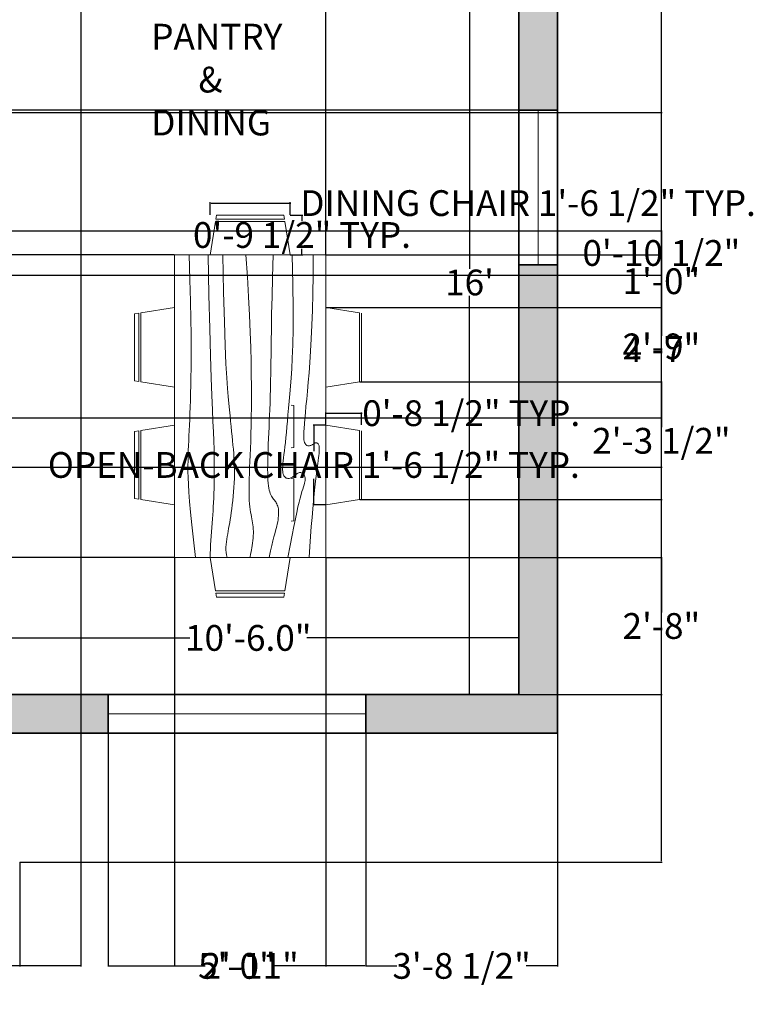
# Model space of a CAD drawing. Units: inches. Extents: x 1174 to 1615, y 3112 to 3628.
# Tile 2 of 6: x 1439 to 1610, y 3112 to 3341. Entities that reach past the tile are written whole.
import ezdxf

# ---------------------------------------------------------------- set-up
doc = ezdxf.new("R2010")
doc.units = ezdxf.units.IN
doc.header["$MEASUREMENT"] = 0
doc.layers.get('0').update_dxf_attribs({"color": 250})
for name, color, linetype, lineweight in [('A-ANNO-DIMS', 2, 'Continuous', 18), ('A-AREA-IDEN', 7, 'Continuous', 25), ('A-FURN', 8, 'Continuous', 13), ('A-GLAZ', 4, 'Continuous', 18), ('A-WALL', 7, 'Continuous', 35)]:
    doc.layers.add(name, color=color, linetype=linetype, lineweight=lineweight)
doc.layers.add('A-WALL-PATT', color=18, linetype='Continuous', lineweight=13, true_color=0x000000)
doc.styles.get("Standard").update_dxf_attribs({"font": 'arial.ttf'})
doc.dimstyles.get("Standard").update_dxf_attribs({"dimtxt": 6, "dimasz": 0.18, "dimexe": 0.18, "dimexo": 0.0625, "dimgap": 0.09, "dimtad": 0, "dimtih": 1, "dimtoh": 1, "dimdec": 1, "dimzin": 0, "dimdsep": 46, "dimlunit": 3, "dimtxsty": 'Standard', "dimcen": 0.09, "dimadec": 0, "dimazin": 0, "dimtfac": 1, "dimtdec": 1, "dimtofl": 0, "dimtmove": 0, "dimatfit": 3, "dimfxl": 1, "dimtolj": 1, "dimtzin": 0, "dimarcsym": 0})

# ---------------------------------------------------------------- blocks, each defined once
blk = doc.blocks.new('*D11')
at = {"layer": 'A-ANNO-DIMS', "color": 0, "lineweight": -2, "transparency": 16777216}
for p, q in [((1429.66, 3184.09), (1429.66, 3197.41)), ((1555.66, 3184.09), (1555.66, 3197.41)), ((1429.84, 3197.23), (1479.05, 3197.23)), ((1555.48, 3197.23), (1506.27, 3197.23))]:
    blk.add_line(p, q, dxfattribs=at)
at = {"layer": 'A-ANNO-DIMS', "color": 0, "transparency": 16777216}
for points in [[(1429.84, 3197.26), (1429.84, 3197.2), (1429.66, 3197.23)], [(1555.48, 3197.26), (1555.48, 3197.2), (1555.66, 3197.23)]]:
    blk.add_solid(points, dxfattribs=at)
at = {"layer": 'Defpoints', "color": 0, "transparency": 16777216}
for p in [(1555.66, 3197.23), (1429.66, 3184.03), (1555.66, 3184.03)]:
    blk.add_point(p, dxfattribs=at)
at = {"layer": 'A-ANNO-DIMS', "color": 0, "transparency": 16777216, "insert": (1492.66, 3197.23), "char_height": 6, "attachment_point": 5}
blk.add_mtext('\\A1;10\'-6.0"', dxfattribs=at)
blk = doc.blocks.new('*D12')
at = {"layer": 'A-ANNO-DIMS', "color": 0, "lineweight": -2, "transparency": 16777216}
for p, q in [((1555.6, 3376.03), (1544, 3376.03)), ((1544.18, 3375.85), (1544.18, 3283.18)), ((1544.18, 3184.21), (1544.18, 3276.88)), ((1555.6, 3184.03), (1544, 3184.03))]:
    blk.add_line(p, q, dxfattribs=at)
at = {"layer": 'A-ANNO-DIMS', "color": 0, "transparency": 16777216}
for points in [[(1544.15, 3375.85), (1544.21, 3375.85), (1544.18, 3376.03)], [(1544.15, 3184.21), (1544.21, 3184.21), (1544.18, 3184.03)]]:
    blk.add_solid(points, dxfattribs=at)
at = {"layer": 'Defpoints', "color": 0, "transparency": 16777216}
for p in [(1555.66, 3376.03), (1544.18, 3184.03), (1555.66, 3184.03)]:
    blk.add_point(p, dxfattribs=at)
at = {"layer": 'A-ANNO-DIMS', "color": 0, "transparency": 16777216, "insert": (1544.18, 3280.03), "char_height": 6, "attachment_point": 5}
blk.add_mtext("\\A1;16'", dxfattribs=at)
blk = doc.blocks.new('WINDOW-36IN')
for p, q in [((-4.5, -36), (-4.5, 0)), ((0, 0), (0, -36)), ((4.5, 0), (4.5, -36))]:
    blk.add_line(p, q)
blk = doc.blocks.new('CHAIR-DINING')
for p, q in [((1.47, 17.34), (9.3, 18.56)), ((0, 17.11), (0.98, 17.26)), ((0, 17.11), (0, 1.45)), ((0.98, 1.3), (0.98, 17.26)), ((1.47, 17.33), (1.47, 1.22)), ((0.98, 1.3), (0, 1.45)), ((9.3, 0), (1.47, 1.22))]:
    blk.add_line(p, q)
blk = doc.blocks.new('CHAIR-DINING-OPEN-BACK')
for p, q in [((7.83, 17.34), (0, 18.56)), ((7.83, 17.33), (7.83, 1.22)), ((8.32, 1.3), (8.32, 17.26)), ((0, 0), (7.83, 1.22))]:
    blk.add_line(p, q)
blk = doc.blocks.new('*D32')
at = {"layer": 'A-ANNO-DIMS', "color": 0, "lineweight": -2, "transparency": 16777216}
for p, q in [((1483.83, 3295.8), (1483.83, 3298.7)), ((1484.01, 3298.52), (1502.21, 3298.52)), ((1502.39, 3295.8), (1502.39, 3298.7)), ((1502.39, 3298.52), (1502.57, 3298.52))]:
    blk.add_line(p, q, dxfattribs=at)
at = {"layer": 'A-ANNO-DIMS', "color": 0, "transparency": 16777216}
for points in [[(1484.01, 3298.55), (1484.01, 3298.49), (1483.83, 3298.52)], [(1502.21, 3298.55), (1502.21, 3298.49), (1502.39, 3298.52)]]:
    blk.add_solid(points, dxfattribs=at)
at = {"layer": 'Defpoints', "color": 0, "transparency": 16777216}
for p in [(1502.39, 3298.52), (1483.83, 3295.73), (1502.39, 3295.73)]:
    blk.add_point(p, dxfattribs=at)
at = {"layer": 'A-ANNO-DIMS', "color": 0, "transparency": 16777216, "insert": (1557.82, 3298.52), "char_height": 6, "attachment_point": 5}
blk.add_mtext('\\A1;DINING CHAIR 1\'-6 1/2" TYP.', dxfattribs=at)
blk = doc.blocks.new('*D33')
at = {"layer": 'A-ANNO-DIMS', "color": 0, "lineweight": -2, "transparency": 16777216}
for p, q in [((1502.45, 3295.73), (1505.35, 3295.73)), ((1505.17, 3295.55), (1505.17, 3294.28)), ((1505.17, 3286.62), (1505.17, 3287.89)), ((1502.45, 3286.44), (1505.35, 3286.44))]:
    blk.add_line(p, q, dxfattribs=at)
at = {"layer": 'A-ANNO-DIMS', "color": 0, "transparency": 16777216}
for points in [[(1505.14, 3295.55), (1505.2, 3295.55), (1505.17, 3295.73)], [(1505.14, 3286.62), (1505.2, 3286.62), (1505.17, 3286.44)]]:
    blk.add_solid(points, dxfattribs=at)
at = {"layer": 'Defpoints', "color": 0, "transparency": 16777216}
for p in [(1502.39, 3295.73), (1502.39, 3286.44), (1505.17, 3286.44)]:
    blk.add_point(p, dxfattribs=at)
at = {"layer": 'A-ANNO-DIMS', "color": 0, "transparency": 16777216, "insert": (1505.17, 3291.09), "char_height": 6, "attachment_point": 5}
blk.add_mtext('\\A1;0\'-9 1/2" TYP.', dxfattribs=at)
blk = doc.blocks.new('*D34')
at = {"layer": 'A-ANNO-DIMS', "color": 0, "lineweight": -2, "transparency": 16777216}
for p, q in [((1510.65, 3246.8), (1507.75, 3246.8)), ((1507.93, 3246.62), (1507.93, 3240.71)), ((1507.93, 3228.42), (1507.93, 3234.32)), ((1510.65, 3228.24), (1507.75, 3228.24))]:
    blk.add_line(p, q, dxfattribs=at)
at = {"layer": 'A-ANNO-DIMS', "color": 0, "transparency": 16777216}
for points in [[(1507.9, 3246.62), (1507.96, 3246.62), (1507.93, 3246.8)], [(1507.9, 3228.42), (1507.96, 3228.42), (1507.93, 3228.24)]]:
    blk.add_solid(points, dxfattribs=at)
at = {"layer": 'Defpoints', "color": 0, "transparency": 16777216}
for p in [(1507.93, 3246.8), (1510.72, 3246.8), (1510.72, 3228.24)]:
    blk.add_point(p, dxfattribs=at)
at = {"layer": 'A-ANNO-DIMS', "color": 0, "transparency": 16777216, "insert": (1507.93, 3237.52), "char_height": 6, "attachment_point": 5}
blk.add_mtext('\\A1;OPEN-BACK CHAIR 1\'-6 1/2" TYP.', dxfattribs=at)
blk = doc.blocks.new('*D35')
at = {"layer": 'A-ANNO-DIMS', "color": 0, "lineweight": -2, "transparency": 16777216}
for p, q in [((1510.72, 3246.86), (1510.72, 3249.76)), ((1510.9, 3249.58), (1518.86, 3249.58)), ((1519.04, 3246.86), (1519.04, 3249.76)), ((1519.04, 3249.58), (1519.22, 3249.58))]:
    blk.add_line(p, q, dxfattribs=at)
at = {"layer": 'A-ANNO-DIMS', "color": 0, "transparency": 16777216}
for points in [[(1510.9, 3249.61), (1510.9, 3249.55), (1510.72, 3249.58)], [(1518.86, 3249.61), (1518.86, 3249.55), (1519.04, 3249.58)]]:
    blk.add_solid(points, dxfattribs=at)
at = {"layer": 'Defpoints', "color": 0, "transparency": 16777216}
for p in [(1519.04, 3249.58), (1510.72, 3246.8), (1519.04, 3246.8)]:
    blk.add_point(p, dxfattribs=at)
at = {"layer": 'A-ANNO-DIMS', "color": 0, "transparency": 16777216, "insert": (1544.58, 3249.58), "char_height": 6, "attachment_point": 5}
blk.add_mtext('\\A1;0\'-8 1/2" TYP.', dxfattribs=at)
blk = doc.blocks.new('*D40')
at = {"layer": 'A-ANNO-DIMS', "color": 0, "lineweight": -2, "transparency": 16777216}
for p, q in [((1342.8, 3144.97), (1342.8, 3120.65)), ((1439.45, 3144.97), (1439.45, 3120.65)), ((1342.98, 3120.83), (1376.07, 3120.83)), ((1439.27, 3120.83), (1406.19, 3120.83))]:
    blk.add_line(p, q, dxfattribs=at)
at = {"layer": 'A-ANNO-DIMS', "color": 0, "transparency": 16777216}
for points in [[(1342.98, 3120.86), (1342.98, 3120.8), (1342.8, 3120.83)], [(1439.27, 3120.86), (1439.27, 3120.8), (1439.45, 3120.83)]]:
    blk.add_solid(points, dxfattribs=at)
at = {"layer": 'Defpoints', "color": 0, "transparency": 16777216}
for p in [(1342.8, 3145.03), (1439.45, 3145.03), (1439.45, 3120.83)]:
    blk.add_point(p, dxfattribs=at)
at = {"layer": 'A-ANNO-DIMS', "color": 0, "transparency": 16777216, "insert": (1391.13, 3120.83), "char_height": 6, "attachment_point": 5}
blk.add_mtext('\\A1;8\'-0 1/2"', dxfattribs=at)
blk = doc.blocks.new('*D41')
at = {"layer": 'A-ANNO-DIMS', "color": 0, "lineweight": -2, "transparency": 16777216}
for p, q in [((1564.73, 3595.03), (1589.04, 3595.03)), ((1588.86, 3594.85), (1588.86, 3373.18)), ((1588.86, 3145.21), (1588.86, 3366.87)), ((1439.51, 3145.03), (1589.04, 3145.03))]:
    blk.add_line(p, q, dxfattribs=at)
at = {"layer": 'A-ANNO-DIMS', "color": 0, "transparency": 16777216}
for points in [[(1588.83, 3594.85), (1588.89, 3594.85), (1588.86, 3595.03)], [(1588.83, 3145.21), (1588.89, 3145.21), (1588.86, 3145.03)]]:
    blk.add_solid(points, dxfattribs=at)
at = {"layer": 'Defpoints', "color": 0, "transparency": 16777216}
for p in [(1564.66, 3595.03), (1588.86, 3595.03), (1439.45, 3145.03)]:
    blk.add_point(p, dxfattribs=at)
at = {"layer": 'A-ANNO-DIMS', "color": 0, "transparency": 16777216, "insert": (1588.86, 3370.03), "char_height": 6, "attachment_point": 5}
blk.add_mtext('\\A1;37\'-6"', dxfattribs=at)
blk = doc.blocks.new('*D44')
at = {"layer": 'A-ANNO-DIMS', "color": 0, "lineweight": -2, "transparency": 16777216}
for p, q in [((1460.02, 3174.97), (1460.02, 3120.65)), ((1520.02, 3174.97), (1520.02, 3120.65)), ((1460.2, 3120.83), (1481.95, 3120.83)), ((1519.84, 3120.83), (1498.08, 3120.83))]:
    blk.add_line(p, q, dxfattribs=at)
at = {"layer": 'A-ANNO-DIMS', "color": 0, "transparency": 16777216}
for points in [[(1460.2, 3120.86), (1460.2, 3120.8), (1460.02, 3120.83)], [(1519.84, 3120.86), (1519.84, 3120.8), (1520.02, 3120.83)]]:
    blk.add_solid(points, dxfattribs=at)
at = {"layer": 'Defpoints', "color": 0, "transparency": 16777216}
for p in [(1460.02, 3175.03), (1520.02, 3175.03), (1520.02, 3120.83)]:
    blk.add_point(p, dxfattribs=at)
at = {"layer": 'A-ANNO-DIMS', "color": 0, "transparency": 16777216, "insert": (1490.02, 3120.83), "char_height": 6, "attachment_point": 5}
blk.add_mtext('\\A1;5\'-0"', dxfattribs=at)
blk = doc.blocks.new('*D45')
at = {"layer": 'A-ANNO-DIMS', "color": 0, "lineweight": -2, "transparency": 16777216}
for p, q in [((1520.02, 3174.97), (1520.02, 3120.65)), ((1564.66, 3174.97), (1564.66, 3120.65)), ((1520.2, 3120.83), (1527.29, 3120.83)), ((1564.48, 3120.83), (1557.39, 3120.83))]:
    blk.add_line(p, q, dxfattribs=at)
at = {"layer": 'A-ANNO-DIMS', "color": 0, "transparency": 16777216}
for points in [[(1520.2, 3120.86), (1520.2, 3120.8), (1520.02, 3120.83)], [(1564.48, 3120.86), (1564.48, 3120.8), (1564.66, 3120.83)]]:
    blk.add_solid(points, dxfattribs=at)
at = {"layer": 'Defpoints', "color": 0, "transparency": 16777216}
for p in [(1520.02, 3175.03), (1564.66, 3175.03), (1564.66, 3120.83)]:
    blk.add_point(p, dxfattribs=at)
at = {"layer": 'A-ANNO-DIMS', "color": 0, "transparency": 16777216, "insert": (1542.34, 3120.83), "char_height": 6, "attachment_point": 5}
blk.add_mtext('\\A1;3\'-8 1/2"', dxfattribs=at)
blk = doc.blocks.new('*D49')
at = {"layer": 'A-ANNO-DIMS', "color": 0, "lineweight": -2, "transparency": 16777216}
for p, q in [((1225.73, 3376.03), (1589.04, 3376.03)), ((1588.86, 3375.85), (1588.86, 3351.02)), ((1588.86, 3319.81), (1588.86, 3344.64)), ((1225.73, 3319.63), (1589.04, 3319.63))]:
    blk.add_line(p, q, dxfattribs=at)
at = {"layer": 'A-ANNO-DIMS', "color": 0, "transparency": 16777216}
for points in [[(1588.83, 3375.85), (1588.89, 3375.85), (1588.86, 3376.03)], [(1588.83, 3319.81), (1588.89, 3319.81), (1588.86, 3319.63)]]:
    blk.add_solid(points, dxfattribs=at)
at = {"layer": 'Defpoints', "color": 0, "transparency": 16777216}
for p in [(1225.66, 3376.03), (1225.66, 3319.63), (1588.86, 3319.63)]:
    blk.add_point(p, dxfattribs=at)
at = {"layer": 'A-ANNO-DIMS', "color": 0, "transparency": 16777216, "insert": (1588.86, 3347.83), "char_height": 6, "attachment_point": 5}
blk.add_mtext('\\A1;4\'-8 1/2"', dxfattribs=at)
blk = doc.blocks.new('*D52')
at = {"layer": 'A-ANNO-DIMS', "color": 0, "lineweight": -2, "transparency": 16777216}
for p, q in [((1555.6, 3376.03), (1192.28, 3376.03)), ((1192.46, 3375.85), (1192.46, 3351.26)), ((1192.46, 3320.35), (1192.46, 3344.95)), ((1555.6, 3320.17), (1192.28, 3320.17))]:
    blk.add_line(p, q, dxfattribs=at)
at = {"layer": 'A-ANNO-DIMS', "color": 0, "transparency": 16777216}
for points in [[(1192.43, 3375.85), (1192.49, 3375.85), (1192.46, 3376.03)], [(1192.43, 3320.35), (1192.49, 3320.35), (1192.46, 3320.17)]]:
    blk.add_solid(points, dxfattribs=at)
at = {"layer": 'Defpoints', "color": 0, "transparency": 16777216}
for p in [(1555.66, 3376.03), (1192.46, 3320.17), (1555.66, 3320.17)]:
    blk.add_point(p, dxfattribs=at)
at = {"layer": 'A-ANNO-DIMS', "color": 0, "transparency": 16777216, "insert": (1192.46, 3348.1), "char_height": 6, "attachment_point": 5}
blk.add_mtext('\\A1;4\'-8"', dxfattribs=at)
blk = doc.blocks.new('*D61')
at = {"layer": 'A-ANNO-DIMS', "color": 0, "lineweight": -2, "transparency": 16777216}
for p, q in [((1252.014815, 3292.048747), (1589.043286, 3292.048747)), ((1588.863286, 3291.868747), (1588.863286, 3267.616767)), ((1588.863286, 3237.184787), (1588.863286, 3261.436767)), ((1252.014815, 3237.004787), (1589.043286, 3237.004787))]:
    blk.add_line(p, q, dxfattribs=at)
at = {"layer": 'A-ANNO-DIMS', "color": 0, "transparency": 16777216}
for points in [[(1588.833286, 3291.868747), (1588.893286, 3291.868747), (1588.863286, 3292.048747)], [(1588.833286, 3237.184787), (1588.893286, 3237.184787), (1588.863286, 3237.004787)]]:
    blk.add_solid(points, dxfattribs=at)
at = {"layer": 'Defpoints', "color": 0, "transparency": 16777216}
for p in [(1251.952315, 3292.048747), (1251.952315, 3237.004787), (1588.863286, 3237.004787)]:
    blk.add_point(p, dxfattribs=at)
at = {"layer": 'A-ANNO-DIMS', "color": 0, "transparency": 16777216, "insert": (1588.863286, 3264.526767), "char_height": 6, "attachment_point": 5}
blk.add_mtext('\\A1;4\'-7"', dxfattribs=at)
blk = doc.blocks.new('*D63')
at = {"layer": 'A-ANNO-DIMS', "color": 0, "lineweight": -2, "transparency": 16777216}
for p, q in [((1285.77, 3281.75), (1589.04, 3281.75)), ((1588.86, 3281.57), (1588.86, 3268.3)), ((1588.86, 3248.71), (1588.86, 3261.99)), ((1285.77, 3248.53), (1589.04, 3248.53))]:
    blk.add_line(p, q, dxfattribs=at)
at = {"layer": 'A-ANNO-DIMS', "color": 0, "transparency": 16777216}
for points in [[(1588.83, 3281.57), (1588.89, 3281.57), (1588.86, 3281.75)], [(1588.83, 3248.71), (1588.89, 3248.71), (1588.86, 3248.53)]]:
    blk.add_solid(points, dxfattribs=at)
at = {"layer": 'Defpoints', "color": 0, "transparency": 16777216}
for p in [(1285.7, 3281.75), (1285.7, 3248.53), (1588.86, 3248.53)]:
    blk.add_point(p, dxfattribs=at)
at = {"layer": 'A-ANNO-DIMS', "color": 0, "transparency": 16777216, "insert": (1588.86, 3265.14), "char_height": 6, "attachment_point": 5}
blk.add_mtext('\\A1;2\'-9"', dxfattribs=at)
blk = doc.blocks.new('*D65')
at = {"layer": 'A-ANNO-DIMS', "color": 0, "lineweight": -2, "transparency": 16777216}
for p, q in [((1252.01, 3292.05), (1589.04, 3292.05)), ((1588.86, 3291.87), (1588.86, 3290.09)), ((1588.86, 3281.93), (1588.86, 3283.71)), ((1269.63, 3281.75), (1589.04, 3281.75))]:
    blk.add_line(p, q, dxfattribs=at)
at = {"layer": 'A-ANNO-DIMS', "color": 0, "transparency": 16777216}
for points in [[(1588.83, 3291.87), (1588.89, 3291.87), (1588.86, 3292.05)], [(1588.83, 3281.93), (1588.89, 3281.93), (1588.86, 3281.75)]]:
    blk.add_solid(points, dxfattribs=at)
at = {"layer": 'Defpoints', "color": 0, "transparency": 16777216}
for p in [(1251.95, 3292.05), (1588.86, 3292.05), (1269.57, 3281.75)]:
    blk.add_point(p, dxfattribs=at)
at = {"layer": 'A-ANNO-DIMS', "color": 0, "transparency": 16777216, "insert": (1588.86, 3286.9), "char_height": 6, "attachment_point": 5}
blk.add_mtext('\\A1;0\'-10 1/2"', dxfattribs=at)
blk = doc.blocks.new('*D66')
at = {"layer": 'A-ANNO-DIMS', "color": 0, "lineweight": -2, "transparency": 16777216}
for p, q in [((1475.5, 3215.93), (1475.5, 3120.65)), ((1510.72, 3215.93), (1510.72, 3120.65)), ((1475.68, 3120.83), (1482.66, 3120.83)), ((1510.54, 3120.83), (1503.55, 3120.83))]:
    blk.add_line(p, q, dxfattribs=at)
at = {"layer": 'A-ANNO-DIMS', "color": 0, "transparency": 16777216}
for points in [[(1475.68, 3120.86), (1475.68, 3120.8), (1475.5, 3120.83)], [(1510.54, 3120.86), (1510.54, 3120.8), (1510.72, 3120.83)]]:
    blk.add_solid(points, dxfattribs=at)
at = {"layer": 'Defpoints', "color": 0, "transparency": 16777216}
for p in [(1475.5, 3215.99), (1510.72, 3215.99), (1510.72, 3120.83)]:
    blk.add_point(p, dxfattribs=at)
at = {"layer": 'A-ANNO-DIMS', "color": 0, "transparency": 16777216, "insert": (1493.11, 3120.83), "char_height": 6, "attachment_point": 5}
blk.add_mtext('\\A1;2\'-11"', dxfattribs=at)
blk = doc.blocks.new('*D67')
at = {"layer": 'A-ANNO-DIMS', "color": 0, "lineweight": -2, "transparency": 16777216}
for p, q in [((1475.43, 3286.44), (1192.28, 3286.44)), ((1192.46, 3286.26), (1192.46, 3254.41)), ((1192.46, 3216.17), (1192.46, 3248.02)), ((1475.43, 3215.99), (1192.28, 3215.99))]:
    blk.add_line(p, q, dxfattribs=at)
at = {"layer": 'A-ANNO-DIMS', "color": 0, "transparency": 16777216}
for points in [[(1192.43, 3286.26), (1192.49, 3286.26), (1192.46, 3286.44)], [(1192.43, 3216.17), (1192.49, 3216.17), (1192.46, 3215.99)]]:
    blk.add_solid(points, dxfattribs=at)
at = {"layer": 'Defpoints', "color": 0, "transparency": 16777216}
for p in [(1475.5, 3286.44), (1192.46, 3215.99), (1475.5, 3215.99)]:
    blk.add_point(p, dxfattribs=at)
at = {"layer": 'A-ANNO-DIMS', "color": 0, "transparency": 16777216, "insert": (1192.46, 3251.22), "char_height": 6, "attachment_point": 5}
blk.add_mtext('\\A1;5\'-10 1/2"', dxfattribs=at)
blk = doc.blocks.new('*D68')
at = {"layer": 'A-ANNO-DIMS', "color": 0, "lineweight": -2, "transparency": 16777216}
for p, q in [((1518.61, 3256.85), (1589.04, 3256.85)), ((1588.86, 3256.67), (1588.86, 3246.35)), ((1588.86, 3229.64), (1588.86, 3239.96)), ((1518.61, 3229.46), (1589.04, 3229.46))]:
    blk.add_line(p, q, dxfattribs=at)
at = {"layer": 'A-ANNO-DIMS', "color": 0, "transparency": 16777216}
for points in [[(1588.83, 3256.67), (1588.89, 3256.67), (1588.86, 3256.85)], [(1588.83, 3229.64), (1588.89, 3229.64), (1588.86, 3229.46)]]:
    blk.add_solid(points, dxfattribs=at)
at = {"layer": 'Defpoints', "color": 0, "transparency": 16777216}
for p in [(1518.55, 3256.85), (1518.55, 3229.46), (1588.86, 3229.46)]:
    blk.add_point(p, dxfattribs=at)
at = {"layer": 'A-ANNO-DIMS', "color": 0, "transparency": 16777216, "insert": (1588.86, 3243.15), "char_height": 6, "attachment_point": 5}
blk.add_mtext('\\A1;2\'-3 1/2"', dxfattribs=at)
blk = doc.blocks.new('*D70')
at = {"layer": 'A-ANNO-DIMS', "color": 0, "lineweight": -2, "transparency": 16777216}
for p, q in [((1390.66, 3585.97), (1390.66, 3120.65)), ((1453.68, 3583.03), (1453.68, 3120.65)), ((1390.84, 3120.83), (1414.11, 3120.83)), ((1453.5, 3120.83), (1430.24, 3120.83))]:
    blk.add_line(p, q, dxfattribs=at)
at = {"layer": 'A-ANNO-DIMS', "color": 0, "transparency": 16777216}
for points in [[(1390.84, 3120.86), (1390.84, 3120.8), (1390.66, 3120.83)], [(1453.5, 3120.86), (1453.5, 3120.8), (1453.68, 3120.83)]]:
    blk.add_solid(points, dxfattribs=at)
at = {"layer": 'Defpoints', "color": 0, "transparency": 16777216}
for p in [(1390.66, 3586.03), (1453.68, 3583.1), (1453.68, 3120.83)]:
    blk.add_point(p, dxfattribs=at)
at = {"layer": 'A-ANNO-DIMS', "color": 0, "transparency": 16777216, "insert": (1422.17, 3120.83), "char_height": 6, "attachment_point": 5}
blk.add_mtext('\\A1;5\'-3"', dxfattribs=at)
blk = doc.blocks.new('*D73')
at = {"layer": 'A-ANNO-DIMS', "color": 0, "lineweight": -2, "transparency": 16777216}
for p, q in [((1510.72, 3286.5), (1510.72, 3619.41)), ((1555.66, 3284.24), (1555.66, 3619.41)), ((1510.9, 3619.23), (1525.13, 3619.23)), ((1555.48, 3619.23), (1541.25, 3619.23))]:
    blk.add_line(p, q, dxfattribs=at)
at = {"layer": 'A-ANNO-DIMS', "color": 0, "transparency": 16777216}
for points in [[(1510.9, 3619.26), (1510.9, 3619.2), (1510.72, 3619.23)], [(1555.48, 3619.26), (1555.48, 3619.2), (1555.66, 3619.23)]]:
    blk.add_solid(points, dxfattribs=at)
at = {"layer": 'Defpoints', "color": 0, "transparency": 16777216}
for p in [(1510.72, 3619.23), (1510.72, 3286.44), (1555.66, 3284.17)]:
    blk.add_point(p, dxfattribs=at)
at = {"layer": 'A-ANNO-DIMS', "color": 0, "transparency": 16777216, "insert": (1533.19, 3619.23), "char_height": 6, "attachment_point": 5}
blk.add_mtext('\\A1;3\'-9"', dxfattribs=at)
blk = doc.blocks.new('*D74')
at = {"layer": 'A-ANNO-DIMS', "color": 0, "lineweight": -2, "transparency": 16777216}
for p, q in [((1510.78, 3215.99), (1589.04, 3215.99)), ((1588.86, 3215.81), (1588.86, 3203.16)), ((1588.86, 3184.21), (1588.86, 3196.86)), ((1520.08, 3184.03), (1589.04, 3184.03))]:
    blk.add_line(p, q, dxfattribs=at)
at = {"layer": 'A-ANNO-DIMS', "color": 0, "transparency": 16777216}
for points in [[(1588.83, 3215.81), (1588.89, 3215.81), (1588.86, 3215.99)], [(1588.83, 3184.21), (1588.89, 3184.21), (1588.86, 3184.03)]]:
    blk.add_solid(points, dxfattribs=at)
at = {"layer": 'Defpoints', "color": 0, "transparency": 16777216}
for p in [(1510.72, 3215.99), (1520.02, 3184.03), (1588.86, 3184.03)]:
    blk.add_point(p, dxfattribs=at)
at = {"layer": 'A-ANNO-DIMS', "color": 0, "transparency": 16777216, "insert": (1588.86, 3200.01), "char_height": 6, "attachment_point": 5}
blk.add_mtext('\\A1;2\'-8"', dxfattribs=at)
blk = doc.blocks.new('*D75')
at = {"layer": 'A-ANNO-DIMS', "color": 0, "lineweight": -2, "transparency": 16777216}
for p, q in [((1510.78, 3286.44), (1589.04, 3286.44)), ((1588.86, 3286.26), (1588.86, 3283.47)), ((1588.86, 3274.37), (1588.86, 3277.16)), ((1510.78, 3274.19), (1589.04, 3274.19))]:
    blk.add_line(p, q, dxfattribs=at)
at = {"layer": 'A-ANNO-DIMS', "color": 0, "transparency": 16777216}
for points in [[(1588.83, 3286.26), (1588.89, 3286.26), (1588.86, 3286.44)], [(1588.83, 3274.37), (1588.89, 3274.37), (1588.86, 3274.19)]]:
    blk.add_solid(points, dxfattribs=at)
at = {"layer": 'Defpoints', "color": 0, "transparency": 16777216}
for p in [(1510.72, 3286.44), (1510.72, 3274.19), (1588.86, 3274.19)]:
    blk.add_point(p, dxfattribs=at)
at = {"layer": 'A-ANNO-DIMS', "color": 0, "transparency": 16777216, "insert": (1588.86, 3280.32), "char_height": 6, "attachment_point": 5}
blk.add_mtext('\\A1;1\'-0"', dxfattribs=at)

msp = doc.modelspace()

# ---------------------------------------------------------------- hatches: boundary and pattern name
at = {"layer": 'A-WALL-PATT'}
h = msp.add_hatch(color=256, dxfattribs=at)
h.dxf.hatch_style = 1
h.paths.add_polyline_path([(1564.66, 3595.03), (1216.66, 3595.03), (1216.66, 3564.55), (1225.66, 3564.55), (1225.66, 3586.03), (1381.66, 3586.03), (1381.66, 3385.03), (1380.66, 3385.03), (1380.66, 3376.03), (1381.66, 3376.03), (1407.66, 3376.03), (1407.66, 3385.03), (1390.66, 3385.03), (1390.66, 3586.03), (1555.66, 3586.03), (1555.66, 3558.83), (1564.66, 3558.83)])
h.paths.add_polyline_path([(1564.66, 3408.64), (1555.66, 3408.64), (1555.66, 3385.03), (1453.66, 3385.03), (1453.66, 3457.03), (1465.66, 3457.03), (1465.66, 3466.03), (1453.66, 3466.03), (1444.66, 3466.03), (1444.66, 3385.03), (1443.66, 3385.03), (1443.66, 3376.03), (1444.66, 3376.03), (1555.66, 3376.03), (1555.66, 3320.17), (1564.66, 3320.17)])
h.paths.add_polyline_path([(1564.66, 3522.83), (1555.66, 3522.83), (1555.66, 3466.03), (1497.66, 3466.03), (1497.66, 3457.03), (1555.66, 3457.03), (1555.66, 3432.64), (1564.66, 3432.64)], flags=17)
h.paths.add_polyline_path([(1344.66, 3385.03), (1336.66, 3385.03), (1336.66, 3466.03), (1269.66, 3466.03), (1269.66, 3457.03), (1327.66, 3457.03), (1327.66, 3385.03), (1225.66, 3385.03), (1225.66, 3413.31), (1216.66, 3413.31), (1216.66, 3319.63), (1225.66, 3319.63), (1225.66, 3376.03), (1344.66, 3376.03)])
h.paths.add_polyline_path([(1237.66, 3466.03), (1225.66, 3466.03), (1225.66, 3528.55), (1216.66, 3528.55), (1216.66, 3437.31), (1225.66, 3437.31), (1225.66, 3457.03), (1237.66, 3457.03)], flags=17)
h.paths.add_polyline_path([(1265.25, 3184.03), (1225.66, 3184.03), (1225.66, 3283.63), (1216.66, 3283.63), (1216.66, 3175.03), (1265.25, 3175.03)])
h.paths.add_polyline_path([(1372.66, 3184.03), (1360.66, 3184.03), (1360.66, 3268.03), (1376.66, 3268.03), (1376.66, 3277.03), (1360.66, 3277.03), (1360.66, 3313.03), (1351.66, 3313.03), (1351.66, 3184.03), (1301.25, 3184.03), (1301.25, 3175.03), (1372.66, 3175.03)])
h.paths.add_polyline_path([(1460.02, 3184.03), (1429.66, 3184.03), (1429.66, 3277.03), (1408.66, 3277.03), (1408.66, 3268.03), (1420.66, 3268.03), (1420.66, 3184.03), (1408.66, 3184.03), (1408.66, 3175.03), (1460.02, 3175.03)])
h.paths.add_polyline_path([(1564.66, 3284.17), (1555.66, 3284.17), (1555.66, 3184.03), (1520.02, 3184.03), (1520.02, 3175.03), (1564.66, 3175.03)])

# ---------------------------------------------------------------- linework, layer by layer
at = {"layer": 'A-FURN'}
for p, q in [((1475.5, 3286.44), (1475.5, 3215.99)), ((1510.72, 3286.44), (1475.5, 3286.44)), ((1510.72, 3215.99), (1510.72, 3286.44)), ((1503.25, 3251.37), (1502.64, 3251.47)), ((1503.25, 3251.37), (1503.25, 3241.61)), ((1502.64, 3241.52), (1503.25, 3241.61)), ((1503.25, 3234.29), (1502.64, 3234.39)), ((1503.25, 3234.29), (1503.25, 3224.53)), ((1502.64, 3224.44), (1503.25, 3224.53)), ((1475.5, 3215.99), (1510.72, 3215.99))]:
    msp.add_line(p, q, dxfattribs=at)
for points in [[(1478.92, 3286.44), (1479.08, 3280.65), (1479.2, 3275.71), (1479.29, 3271.5), (1479.34, 3267.93), (1479.36, 3264.88), (1479.37, 3262.27), (1479.35, 3259.99), (1479.33, 3257.94), (1479.29, 3256.03), (1479.25, 3254.24), (1479.21, 3252.56), (1479.15, 3250.98), (1479.1, 3249.49), (1479.04, 3248.09), (1478.98, 3246.76), (1478.92, 3245.51), (1478.86, 3244.31), (1478.8, 3243.16), (1478.75, 3242.03), (1478.7, 3240.9), (1478.66, 3239.75), (1478.64, 3238.57), (1478.63, 3237.33), (1478.63, 3236.01), (1478.66, 3234.59), (1478.72, 3233), (1478.82, 3231.18), (1478.98, 3229.04), (1479.2, 3226.53), (1479.5, 3223.56), (1479.89, 3220.07), (1480.39, 3215.99)], [(1483.32, 3286.44), (1483.51, 3277.05), (1483.69, 3269.28), (1483.86, 3262.94), (1484.03, 3257.81), (1484.18, 3253.68), (1484.32, 3250.36), (1484.44, 3247.62), (1484.55, 3245.26), (1484.63, 3243.12), (1484.69, 3241.14), (1484.73, 3239.31), (1484.75, 3237.62), (1484.76, 3236.06), (1484.75, 3234.62), (1484.74, 3233.29), (1484.71, 3232.05), (1484.68, 3230.9), (1484.63, 3229.82), (1484.59, 3228.79), (1484.53, 3227.8), (1484.47, 3226.84), (1484.41, 3225.9), (1484.34, 3224.95), (1484.26, 3223.98), (1484.18, 3222.99), (1484.1, 3221.98), (1484.03, 3220.95), (1483.96, 3219.93), (1483.9, 3218.91), (1483.85, 3217.91), (1483.82, 3216.93), (1483.81, 3215.99)], [(1486.75, 3286.44), (1486.93, 3277.81), (1487.11, 3270.87), (1487.29, 3265.37), (1487.47, 3261.11), (1487.65, 3257.84), (1487.81, 3255.36), (1487.98, 3253.43), (1488.13, 3251.83), (1488.28, 3250.36), (1488.42, 3248.99), (1488.56, 3247.71), (1488.68, 3246.49), (1488.8, 3245.34), (1488.91, 3244.24), (1489.02, 3243.19), (1489.11, 3242.16), (1489.2, 3241.17), (1489.28, 3240.19), (1489.34, 3239.22), (1489.4, 3238.25), (1489.44, 3237.29), (1489.46, 3236.32), (1489.46, 3235.34), (1489.44, 3234.34), (1489.4, 3233.32), (1489.34, 3232.29), (1489.26, 3231.25), (1489.16, 3230.23), (1489.06, 3229.22), (1488.95, 3228.25), (1488.83, 3227.31), (1488.7, 3226.43), (1488.58, 3225.6), (1488.46, 3224.83), (1488.34, 3224.1), (1488.22, 3223.41), (1488.1, 3222.74), (1487.99, 3222.1), (1487.88, 3221.47), (1487.77, 3220.84), (1487.66, 3220.22), (1487.57, 3219.59), (1487.5, 3218.96), (1487.46, 3218.34), (1487.45, 3217.73), (1487.49, 3217.13), (1487.58, 3216.55), (1487.73, 3215.99)], [(1492.13, 3286.44), (1492.46, 3281.34), (1492.73, 3276.67), (1492.95, 3272.4), (1493.11, 3268.49), (1493.23, 3264.91), (1493.32, 3261.64), (1493.37, 3258.63), (1493.39, 3255.86), (1493.4, 3253.3), (1493.39, 3250.93), (1493.36, 3248.74), (1493.33, 3246.7), (1493.28, 3244.8), (1493.23, 3243.03), (1493.17, 3241.37), (1493.11, 3239.8), (1493.05, 3238.31), (1492.99, 3236.9), (1492.94, 3235.56), (1492.89, 3234.31), (1492.86, 3233.13), (1492.84, 3232.04), (1492.84, 3231.03), (1492.86, 3230.1), (1492.9, 3229.25), (1492.96, 3228.48), (1493.04, 3227.78), (1493.13, 3227.13), (1493.22, 3226.54), (1493.32, 3225.98), (1493.42, 3225.46), (1493.52, 3224.96), (1493.6, 3224.48), (1493.68, 3224.01), (1493.75, 3223.54), (1493.8, 3223.07), (1493.84, 3222.59), (1493.86, 3222.09), (1493.86, 3221.58), (1493.84, 3221.05), (1493.8, 3220.48), (1493.74, 3219.91), (1493.67, 3219.33), (1493.59, 3218.77), (1493.5, 3218.24), (1493.42, 3217.76), (1493.34, 3217.35), (1493.27, 3217.01), (1493.22, 3216.76), (1493.18, 3216.59), (1493.15, 3216.48), (1493.13, 3216.39), (1493.12, 3216.33), (1493.11, 3216.25), (1493.11, 3216.14), (1493.11, 3215.99)], [(1498.49, 3286.44), (1498.33, 3281.27), (1498.2, 3276.72), (1498.11, 3272.74), (1498.05, 3269.25), (1498.01, 3266.19), (1497.97, 3263.5), (1497.95, 3261.11), (1497.92, 3258.96), (1497.88, 3257), (1497.84, 3255.19), (1497.8, 3253.51), (1497.74, 3251.94), (1497.69, 3250.46), (1497.63, 3249.04), (1497.57, 3247.67), (1497.51, 3246.32), (1497.45, 3244.98), (1497.39, 3243.65), (1497.34, 3242.34), (1497.29, 3241.06), (1497.24, 3239.84), (1497.21, 3238.66), (1497.19, 3237.56), (1497.18, 3236.54), (1497.19, 3235.61), (1497.21, 3234.76), (1497.25, 3233.99), (1497.31, 3233.31), (1497.38, 3232.69), (1497.46, 3232.15), (1497.56, 3231.66), (1497.67, 3231.24), (1497.8, 3230.87), (1497.94, 3230.54), (1498.1, 3230.25), (1498.25, 3230), (1498.42, 3229.76), (1498.58, 3229.54), (1498.74, 3229.33), (1498.9, 3229.12), (1499.05, 3228.9), (1499.18, 3228.67), (1499.31, 3228.43), (1499.43, 3228.17), (1499.53, 3227.89), (1499.61, 3227.59), (1499.67, 3227.27), (1499.71, 3226.92), (1499.73, 3226.54), (1499.73, 3226.13), (1499.7, 3225.69), (1499.66, 3225.24), (1499.6, 3224.76), (1499.52, 3224.27), (1499.42, 3223.76), (1499.3, 3223.25), (1499.17, 3222.72), (1499.02, 3222.15), (1498.85, 3221.5), (1498.65, 3220.75), (1498.42, 3219.86), (1498.16, 3218.79), (1497.86, 3217.51), (1497.51, 3215.99)], [(1502.89, 3286.44), (1503.03, 3279.57), (1503.09, 3273.89), (1503.09, 3269.24), (1503.02, 3265.47), (1502.92, 3262.41), (1502.79, 3259.9), (1502.64, 3257.79), (1502.48, 3255.9), (1502.34, 3254.12), (1502.19, 3252.41), (1502.06, 3250.78), (1501.92, 3249.23), (1501.8, 3247.76), (1501.67, 3246.38), (1501.55, 3245.08), (1501.42, 3243.88), (1501.3, 3242.76), (1501.18, 3241.73), (1501.07, 3240.79), (1500.97, 3239.93), (1500.87, 3239.15), (1500.79, 3238.45), (1500.73, 3237.83), (1500.69, 3237.27), (1500.67, 3236.79), (1500.67, 3236.36), (1500.7, 3236), (1500.74, 3235.68), (1500.8, 3235.41), (1500.89, 3235.19), (1500.98, 3234.99), (1501.1, 3234.83), (1501.23, 3234.69), (1501.37, 3234.57), (1501.53, 3234.48), (1501.69, 3234.41), (1501.86, 3234.37), (1502.04, 3234.36), (1502.22, 3234.37), (1502.4, 3234.42), (1502.59, 3234.49), (1502.77, 3234.59), (1502.95, 3234.71), (1503.14, 3234.85), (1503.32, 3234.99), (1503.5, 3235.13), (1503.69, 3235.27), (1503.87, 3235.4), (1504.05, 3235.51), (1504.24, 3235.61), (1504.42, 3235.68), (1504.59, 3235.73), (1504.77, 3235.76), (1504.94, 3235.75), (1505.1, 3235.72), (1505.26, 3235.64), (1505.4, 3235.53), (1505.54, 3235.39), (1505.66, 3235.21), (1505.77, 3235), (1505.85, 3234.77), (1505.9, 3234.51), (1505.92, 3234.23), (1505.91, 3233.93), (1505.86, 3233.61), (1505.78, 3233.27), (1505.66, 3232.88), (1505.52, 3232.44), (1505.35, 3231.92), (1505.16, 3231.32), (1504.95, 3230.62), (1504.73, 3229.81), (1504.49, 3228.87), (1504.24, 3227.77), (1503.95, 3226.48), (1503.64, 3224.97), (1503.29, 3223.19), (1502.89, 3221.13), (1502.43, 3218.74), (1501.91, 3215.99)], [(1507.78, 3286.44), (1507.76, 3281.72), (1507.7, 3277.45), (1507.6, 3273.58), (1507.48, 3270.08), (1507.33, 3266.91), (1507.16, 3264.03), (1506.99, 3261.41), (1506.81, 3259), (1506.62, 3256.78), (1506.44, 3254.74), (1506.27, 3252.87), (1506.11, 3251.18), (1505.97, 3249.66), (1505.84, 3248.3), (1505.74, 3247.11), (1505.66, 3246.08), (1505.62, 3245.21), (1505.6, 3244.48), (1505.61, 3243.89), (1505.64, 3243.41), (1505.7, 3243.03), (1505.78, 3242.73), (1505.88, 3242.5), (1505.99, 3242.33), (1506.12, 3242.19), (1506.26, 3242.09), (1506.41, 3242.03), (1506.57, 3241.99), (1506.73, 3241.98), (1506.9, 3242), (1507.06, 3242.03), (1507.21, 3242.08), (1507.36, 3242.15), (1507.51, 3242.23), (1507.64, 3242.31), (1507.77, 3242.4), (1507.9, 3242.48), (1508.03, 3242.55), (1508.15, 3242.61), (1508.27, 3242.65), (1508.4, 3242.67), (1508.52, 3242.67), (1508.63, 3242.64), (1508.74, 3242.59), (1508.84, 3242.52), (1508.94, 3242.42), (1509.02, 3242.31), (1509.09, 3242.16), (1509.14, 3242), (1509.18, 3241.81), (1509.2, 3241.58), (1509.21, 3241.31), (1509.2, 3240.99), (1509.18, 3240.63), (1509.14, 3240.21), (1509.09, 3239.72), (1509.02, 3239.16), (1508.94, 3238.53), (1508.84, 3237.8), (1508.73, 3236.96), (1508.61, 3236.01), (1508.48, 3234.93), (1508.34, 3233.71), (1508.19, 3232.34), (1508.04, 3230.81), (1507.87, 3229.11), (1507.7, 3227.27), (1507.53, 3225.28), (1507.35, 3223.15), (1507.17, 3220.89), (1506.99, 3218.5), (1506.81, 3215.99)]]:
    msp.add_lwpolyline(points, dxfattribs=at)
at = {"layer": 'A-GLAZ'}
for p, q in [((1520.02, 3184.03), (1460.02, 3184.03)), ((1460.02, 3179.53), (1520.02, 3179.53)), ((1460.02, 3175.03), (1520.02, 3175.03))]:
    msp.add_line(p, q, dxfattribs=at)
at = {"layer": 'A-WALL'}
for p, q in [((1564.66, 3595.03), (1564.66, 3175.03)), ((1555.66, 3376.03), (1555.66, 3184.03)), ((1555.66, 3320.17), (1564.66, 3320.17)), ((1564.66, 3284.17), (1555.66, 3284.17)), ((1429.66, 3184.03), (1555.66, 3184.03)), ((1460.02, 3184.03), (1460.02, 3175.03)), ((1520.02, 3175.03), (1520.02, 3184.03)), ((1216.66, 3175.03), (1564.66, 3175.03))]:
    msp.add_line(p, q, dxfattribs=at)

# ---------------------------------------------------------------- block references
at = {"layer": 'A-FURN'}
for p, rotation in [((1483.83, 3295.73), 270.0000441632014), ((1502.39, 3206.7), 89.99413959734574)]:
    msp.add_blockref('CHAIR-DINING', p, dxfattribs=dict(at, rotation=rotation))
for name, p in [('CHAIR-DINING', (1466.2, 3255.63)), ('CHAIR-DINING-OPEN-BACK', (1510.72, 3255.63)), ('CHAIR-DINING', (1466.2, 3228.24)), ('CHAIR-DINING-OPEN-BACK', (1510.72, 3228.24))]:
    msp.add_blockref(name, p, dxfattribs=at)
at = {"layer": 'A-GLAZ', "rotation": 180}
msp.add_blockref('WINDOW-36IN', (1560.16, 3284.17), dxfattribs=at)

# ---------------------------------------------------------------- texts
at = {"layer": 'A-AREA-IDEN', "insert": (1470.08, 3340.29), "char_height": 6, "attachment_point": 1}
msp.add_mtext_dynamic_manual_height_columns('PANTRY\\P      &\\PDINING', width=54.737, gutter_width=1, heights=[0], dxfattribs=at)

# ---------------------------------------------------------------- dimensions: what is measured, and where the dimension line sits
at = {"layer": 'A-ANNO-DIMS'}
for base, p1, p2, override, picture, middle in [((1510.72, 3619.23), (1555.66, 3284.17), (1510.72, 3286.44), {"dimdec": 1, "dimlfac": 1, "dimrnd": 0, "dimzin": 1, "dimdsep": 46, "dimlunit": 4, "dimfrac": 2}, '*D73', (1533.19, 3619.23)), ((1453.68, 3120.83), (1390.66, 3586.03), (1453.68, 3583.1), {"dimdec": 1, "dimlfac": 1, "dimrnd": 0, "dimzin": 1, "dimdsep": 46, "dimlunit": 4, "dimfrac": 2}, '*D70', (1422.17, 3120.83)), ((1510.72, 3120.83), (1475.5, 3215.99), (1510.72, 3215.99), {"dimdec": 1, "dimlfac": 1, "dimrnd": 0, "dimzin": 1, "dimdsep": 46, "dimlunit": 4, "dimfrac": 2}, '*D66', (1493.11, 3120.83)), ((1555.66, 3197.23), (1429.66, 3184.03), (1555.66, 3184.03), {"dimclrd": 0, "dimclre": 0, "dimclrt": 0}, '*D11', (1492.66, 3197.23)), ((1520.02, 3120.83), (1460.02, 3175.03), (1520.02, 3175.03), {"dimdec": 1, "dimlfac": 1, "dimrnd": 0, "dimzin": 1, "dimdsep": 46, "dimlunit": 4, "dimfrac": 2}, '*D44', (1490.02, 3120.83)), ((1564.66, 3120.83), (1520.02, 3175.03), (1564.66, 3175.03), {"dimdec": 1, "dimlfac": 1, "dimrnd": 0, "dimzin": 1, "dimdsep": 46, "dimlunit": 4, "dimfrac": 2}, '*D45', (1542.34, 3120.83)), ((1439.4482, 3120.8288), (1342.8038, 3145.0288), (1439.4482, 3145.0288), {"dimdec": 1, "dimlfac": 1, "dimrnd": 0, "dimzin": 1, "dimdsep": 46, "dimlunit": 4, "dimfrac": 2}, '*D40', (1391.126, 3120.8288))]:
    dim = msp.add_linear_dim(base=base, p1=p1, p2=p2, dimstyle='Standard', override=override, dxfattribs=at)
    dim.commit()
    dim.dimension.update_dxf_attribs({"geometry": picture, "text_midpoint": middle})
for base, p1, p2, override, picture, middle in [((1588.86, 3595.03), (1439.45, 3145.03), (1564.66, 3595.03), {"dimdec": 1, "dimlfac": 1, "dimrnd": 0, "dimzin": 1, "dimdsep": 46, "dimlunit": 4, "dimfrac": 2}, '*D41', (1588.86, 3370.03)), ((1192.46, 3320.17), (1555.66, 3376.03), (1555.66, 3320.17), {"dimdec": 1, "dimlfac": 1, "dimrnd": 0, "dimzin": 1, "dimdsep": 46, "dimlunit": 4, "dimfrac": 2}, '*D52', (1192.46, 3348.1)), ((1588.86, 3319.63), (1225.66, 3376.03), (1225.66, 3319.63), {"dimdec": 1, "dimlfac": 1, "dimrnd": 0, "dimzin": 1, "dimdsep": 46, "dimlunit": 4, "dimfrac": 2}, '*D49', (1588.86, 3347.83)), ((1544.18, 3184.03), (1555.66, 3376.03), (1555.66, 3184.03), {"dimclrd": 0, "dimclre": 0, "dimclrt": 0}, '*D12', (1544.18, 3280.03)), ((1588.86, 3292.05), (1269.57, 3281.75), (1251.95, 3292.05), {"dimdec": 1, "dimlfac": 1, "dimrnd": 0, "dimzin": 1, "dimdsep": 46, "dimlunit": 4, "dimfrac": 2}, '*D65', (1588.86, 3286.9)), ((1588.8633, 3237.0048), (1251.9523, 3292.0487), (1251.9523, 3237.0048), {"dimdec": 1, "dimlfac": 1, "dimrnd": 0, "dimzin": 1, "dimdsep": 46, "dimlunit": 4, "dimfrac": 2}, '*D61', (1588.8633, 3264.5268)), ((1192.4633, 3215.9918), (1475.4958, 3286.439), (1475.4958, 3215.9918), {"dimdec": 1, "dimlfac": 1, "dimrnd": 0, "dimzin": 1, "dimdsep": 46, "dimlunit": 4, "dimfrac": 2}, '*D67', (1192.4633, 3251.2154)), ((1588.8633, 3274.1936), (1510.7194, 3286.439), (1510.717, 3274.1936), {"dimdec": 1, "dimlfac": 1, "dimrnd": 0, "dimzin": 1, "dimdsep": 46, "dimlunit": 4, "dimfrac": 2}, '*D75', (1588.8633, 3280.3163)), ((1588.86, 3248.53), (1285.7, 3281.75), (1285.7, 3248.53), {"dimdec": 1, "dimlfac": 1, "dimrnd": 0, "dimzin": 1, "dimdsep": 46, "dimlunit": 4, "dimfrac": 2}, '*D63', (1588.86, 3265.14)), ((1588.86, 3229.46), (1518.55, 3256.85), (1518.55, 3229.46), {"dimdec": 1, "dimlfac": 1, "dimrnd": 0, "dimzin": 1, "dimdsep": 46, "dimlunit": 4, "dimfrac": 2}, '*D68', (1588.86, 3243.15)), ((1588.86, 3184.03), (1510.72, 3215.99), (1520.02, 3184.03), {"dimdec": 1, "dimlfac": 1, "dimrnd": 0, "dimzin": 1, "dimdsep": 46, "dimlunit": 4, "dimfrac": 2}, '*D74', (1588.86, 3200.01))]:
    dim = msp.add_linear_dim(base=base, p1=p1, p2=p2, angle=90, dimstyle='Standard', override=override, dxfattribs=at)
    dim.commit()
    dim.dimension.update_dxf_attribs({"geometry": picture, "text_midpoint": middle})
for base, p1, p2, angle, text, picture, middle in [((1502.39, 3298.52), (1483.83, 3295.73), (1502.39, 3295.73), 0, 'DINING CHAIR <> TYP.', '*D32', (1557.82, 3298.52)), ((1505.17, 3286.44), (1502.39, 3295.73), (1502.39, 3286.44), 270, '<> TYP.', '*D33', (1505.17, 3291.09)), ((1507.93, 3246.8), (1510.72, 3228.24), (1510.72, 3246.8), 90, 'OPEN-BACK CHAIR <> TYP.', '*D34', (1507.93, 3237.52))]:
    dim = msp.add_linear_dim(base=base, p1=p1, p2=p2, angle=angle, text=text, dimstyle='Standard', override={"dimdec": 1, "dimlfac": 1, "dimrnd": 0, "dimzin": 1, "dimdsep": 46, "dimlunit": 4, "dimfrac": 2}, dxfattribs=at)
    dim.commit()
    dim.dimension.update_dxf_attribs({"geometry": picture, "text_midpoint": middle})
dim = msp.add_linear_dim(base=(1519.04, 3249.58), p1=(1510.72, 3246.8), p2=(1519.04, 3246.8), text='<> TYP.', dimstyle='Standard', override={"dimdec": 1, "dimlfac": 1, "dimrnd": 0, "dimzin": 1, "dimdsep": 46, "dimlunit": 4, "dimfrac": 2}, dxfattribs=at)
dim.commit()
dim.dimension.update_dxf_attribs({"geometry": '*D35', "text_midpoint": (1544.58, 3249.58)})

doc.saveas('drawing.dxf')
